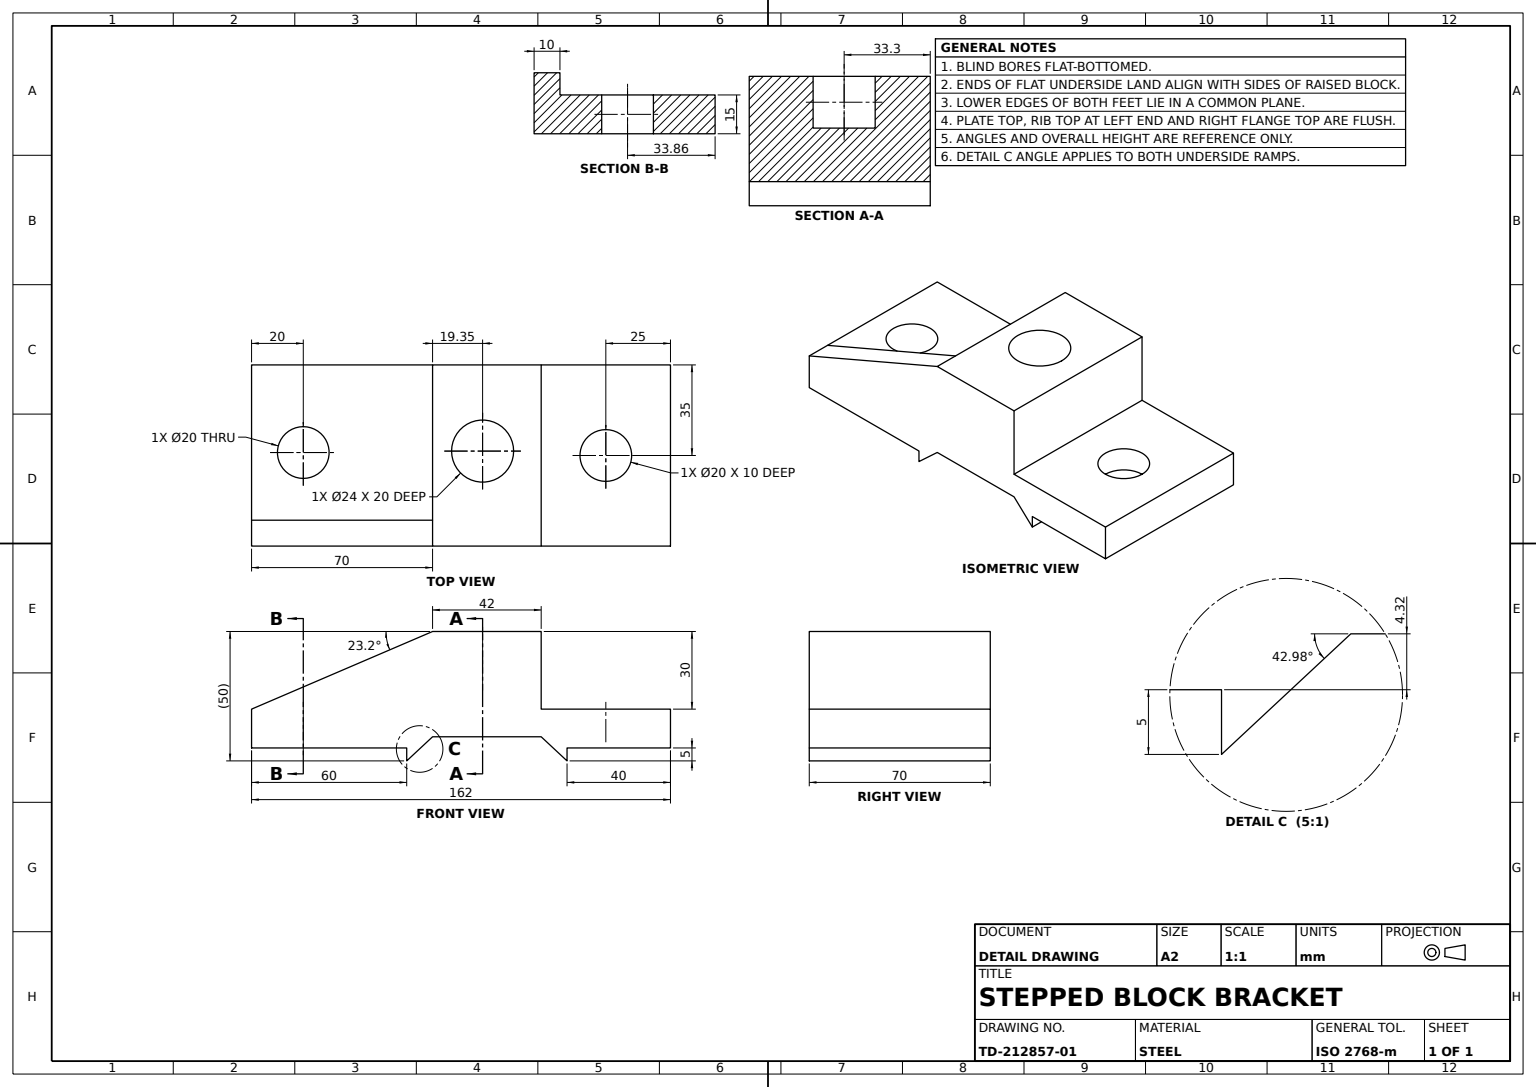
SolidWorks part; units mm, degrees
material "Plain Carbon Steel"
ref_plane "Front Plane" through (0, 0, 0) normal (0, 0, 1) x (1, 0, 0)
ref_plane "Top Plane" through (0, 0, 0) normal (0, 1, 0) x (1, 0, 0)
ref_plane "Right Plane" through (0, 0, 0) normal (1, 0, 0) x (0, 0, -1)
sketch "Stepped Block Profile Sketch" plane through (0, 0, 0) normal (0, 0, 1) x (1, 0, 0)
  line L1 (70, 0) -> (70, -5)
  line L7 (132, -5) -> (132, 0)
  line L8 (132, 0) -> (172, 0)
  line L9 (172, 0) -> (172, 15)
  line L10 (172, 15) -> (122, 15)
  line L11 (122, 15) -> (122, 45)
  line L12 (122, 45) -> (80, 45)
  line L13 (80, 45) -> (80, 15)
  line L22 (70, 0) -> (10, 0)
  line L23 (10, 0) -> (10, 15)
  line L24 (10, 15) -> (80, 15)
  line L27 (80, 4.3191) -> (122, 4.3191)
  line L28 (70, -5) -> (80, 4.3191)
  line L29 (122, 4.3191) -> (132, -5)
  dimension "D2" = 10
  dimension "D3" = 40
  dimension "D4" = 70
  dimension "D5" = 42
  dimension "D6" = 5
  dimension "D7" = 4.3191
  dimension "D8" = 30
  dimension "D9" = 50
  dimension "D11" = 30
  dimension "D12" = 50
extrude "Stepped Block Body" add sketch "Stepped Block Profile Sketch" along normal blind 70
sketch "Hole A Sketch" plane through (0, 15, 0) normal (0, 1, 0) x (1, 0, 0)
  line L1 (80, 0) -> (10, 0) construction
  circle A0 centre (30, -33.8566) radius 10
  dimension "D1" = 20
  dimension "D2" = 20
  dimension "D3" = 33.8566
extrude "Hole A Depth 20" cut sketch "Hole A Sketch" against normal blind 20
sketch "Hole B Sketch" plane through (0, 45, 0) normal (0, 1, 0) x (1, 0, 0)
  line L0 (80, -70) -> (80, 0) construction
  line L1 (122, 0) -> (80, 0) construction
  circle A0 centre (99.3472, -33.2964) radius 12
  dimension "D1" = 24
  dimension "D2" = 19.3472
  dimension "D3" = 33.2964
extrude "Hole B Depth 20" cut sketch "Hole B Sketch" against normal blind 20
sketch "Triangular Lug Sketch" plane through (0, 0, 70) normal (0, 0, 1) x (1, 0, 0)
  line L0 (10, 15) -> (80, 15)
  line L1 (80, 15) -> (80, 45)
  line L2 (122, 45) -> (80, 45) construction
  line L3 (80, 45) -> (80, 15) construction
  line L4 (80, 45) -> (10, 15)
extrude "Triangular Lug" add sketch "Triangular Lug Sketch" against normal blind 10
sketch "Round Boss Sketch" plane through (0, 15, 0) normal (0, 1, 0) x (1, 0, 0)
  line L0 (122, -70) -> (122, 0) construction
  line L1 (172, 0) -> (122, 0) construction
  circle A0 centre (147.5417, -38.1884) radius 10
  dimension "D1" = 20
  dimension "D2" = 25.5417
  dimension "D3" = 38.1884
extrude "Round Boss 10mm" add sketch "Round Boss Sketch" against normal blind 10
sketch "Hole C Sketch" plane through (0, 15, 0) normal (0, 1, 0) x (1, 0, 0)
  line L0 (122, -70) -> (122, 0) construction
  circle A0 centre (147, -35) radius 10
  dimension "D1" = 35
  dimension "D3" = 20
  dimension "D2" = 25
extrude "Hole C Depth 10" cut sketch "Hole C Sketch" against normal blind 10
